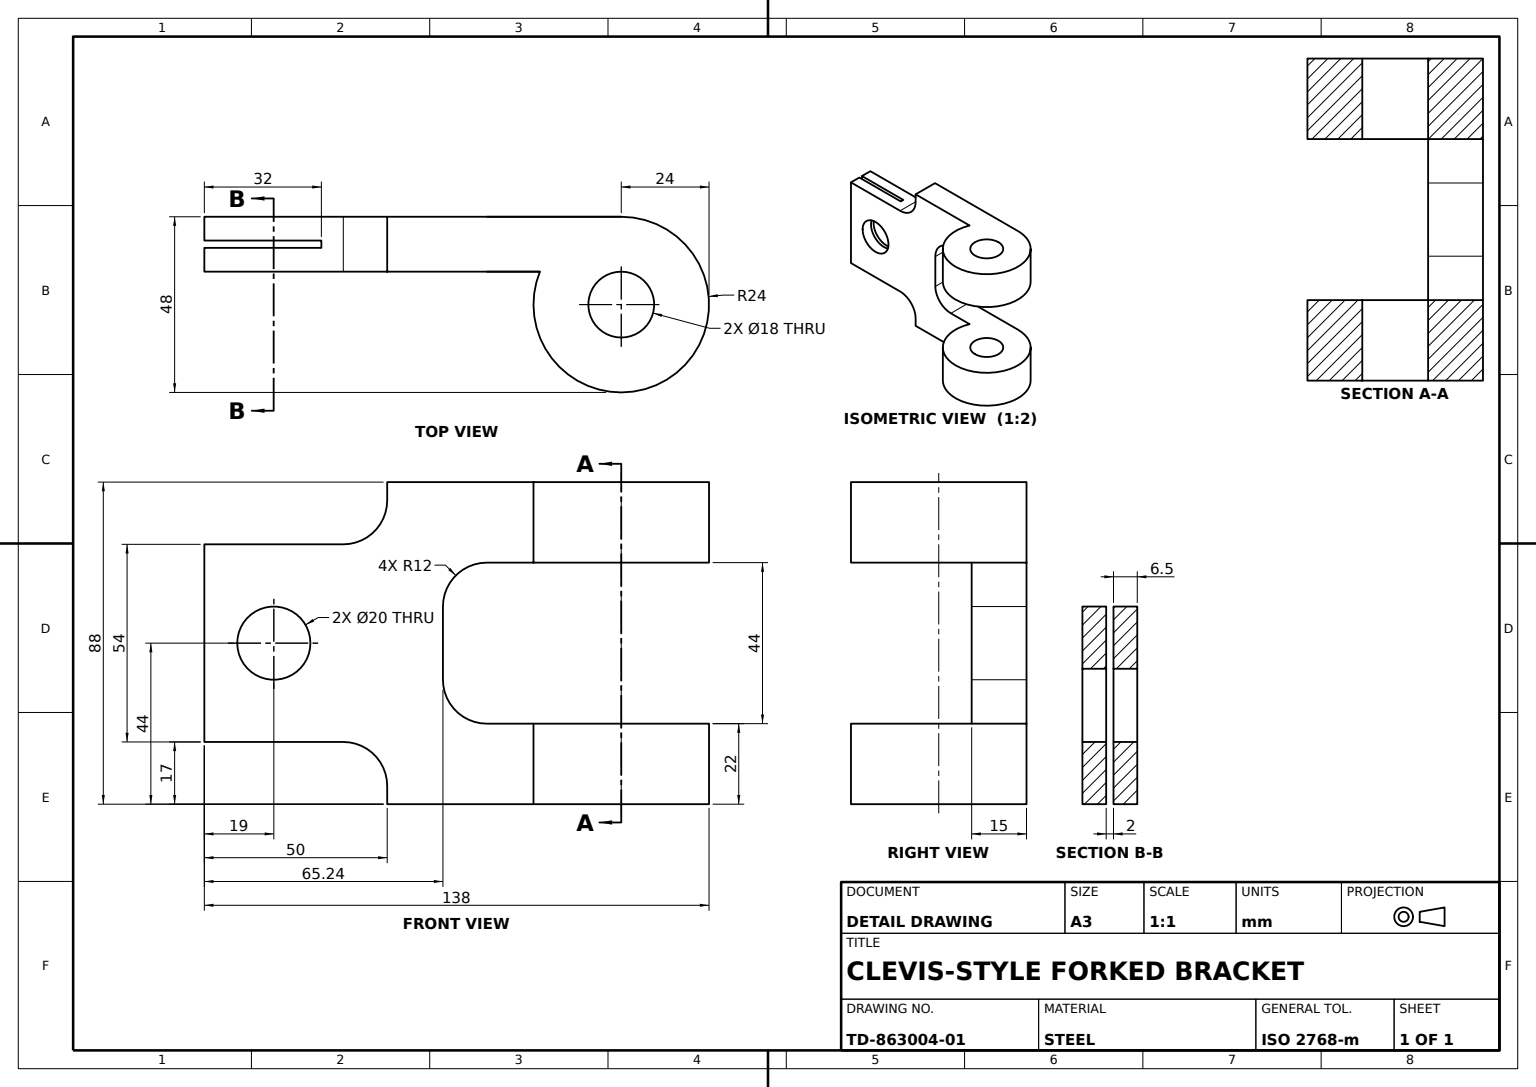
from build123d import *

# Parameters (mm, degrees)
BASE_PLATE_DEPTH         = 15
PIVOT_BOSS_1_PROFILE_R   = 24
PIVOT_BOSS_1_DEPTH       = 22
PIVOT_START              = -22
PIVOT_BOSS_2_PROFILE_R   = 24
PIVOT_BOSS_2_DEPTH       = 22
UPRIGHT_WEB_DEPTH        = 15
WEB_SLOT_DEPTH           = 55
WEB_HOLE_PROFILE_R       = 10
WEB_HOLE_DEPTH           = 55
PIVOT_BORE_PROFILE_R     = 9
PIVOT_BORE_THROUGH_DEPTH = 90


with BuildPart() as part:
    # Base Plate Profile → Base Plate (new body)
    with BuildSketch(Plane.XY):
        with BuildLine():
            Line((0, 0), (64, 0))
            Line((64, 0), (64, -22))
            Line((64, -22), (27.24, -22))
            ThreePointArc((27.24, -22), (18.754718626, -25.514718626), (15.24, -34))
            Line((15.24, -34), (15.24, -54))
            ThreePointArc((15.24, -54), (18.754718626, -62.485281374), (27.24, -66))
            Line((27.24, -66), (64, -66))
            Line((64, -66), (64, -88))
            Line((64, -88), (0, -88))
            Line((0, -88), (0, 0))
        make_face()
    extrude(amount=BASE_PLATE_DEPTH)

    # Pivot Boss 1 Profile → Pivot Boss 1 (add)
    with BuildSketch(Plane(origin=(0, 0, 0), x_dir=(1, 0, 0), z_dir=(0, 1, 0))):
        with Locations((64, -24)):
            Circle(PIVOT_BOSS_1_PROFILE_R)
    extrude(amount=-PIVOT_BOSS_1_DEPTH)

    # Pivot Boss 2 Profile → Pivot Boss 2 (add)
    with BuildSketch(Plane.XZ.offset(88).offset(PIVOT_START)):
        with Locations((64, 24)):
            Circle(PIVOT_BOSS_2_PROFILE_R)
    extrude(amount=PIVOT_BOSS_2_DEPTH)

    # Upright Web Profile → Upright Web (add)
    with BuildSketch(Plane(origin=(0, 0, 0), x_dir=(-1, 0, 0), z_dir=(0, 0, -1))):
        with BuildLine():
            Line((0, -44), (0, -17))
            Line((0, -17), (0, -5))
            ThreePointArc((0, -5), (3.514718626, -13.485281374), (12, -17))
            Line((12, -17), (50, -17))
            Line((50, -17), (50, -71))
            Line((50, -71), (12, -71))
            ThreePointArc((12, -71), (3.514718626, -74.514718626), (0, -83))
            Line((0, -83), (0, -71))
            Line((0, -71), (0, -44))
        make_face()
    extrude(amount=-UPRIGHT_WEB_DEPTH)

    # Web Slot Profile → Web Slot (cut)
    with BuildSketch(Plane(origin=(0, -17, 0), x_dir=(1, 0, 0), z_dir=(0, 1, 0))):
        Polygon((-50, -7.5), (-50, -6.5), (-18, -6.5), (-18, -8.5), (-50, -8.5), align=None)
    extrude(amount=-WEB_SLOT_DEPTH, mode=Mode.SUBTRACT)

    # Web Hole Profile → Web Hole (cut)
    with BuildSketch(Plane.XY.offset(15)):
        with Locations((-31, -44)):
            Circle(WEB_HOLE_PROFILE_R)
    extrude(amount=-WEB_HOLE_DEPTH, mode=Mode.SUBTRACT)

    # Pivot Bore Profile → Pivot Bore Through (cut)
    with BuildSketch(Plane(origin=(0, 0, 0), x_dir=(1, 0, 0), z_dir=(0, 1, 0))):
        with Locations(Location((64, -24, 0), (0, 0, 270))):
            Circle(PIVOT_BORE_PROFILE_R)
    extrude(amount=-PIVOT_BORE_THROUGH_DEPTH, mode=Mode.SUBTRACT)


solid = part.part
